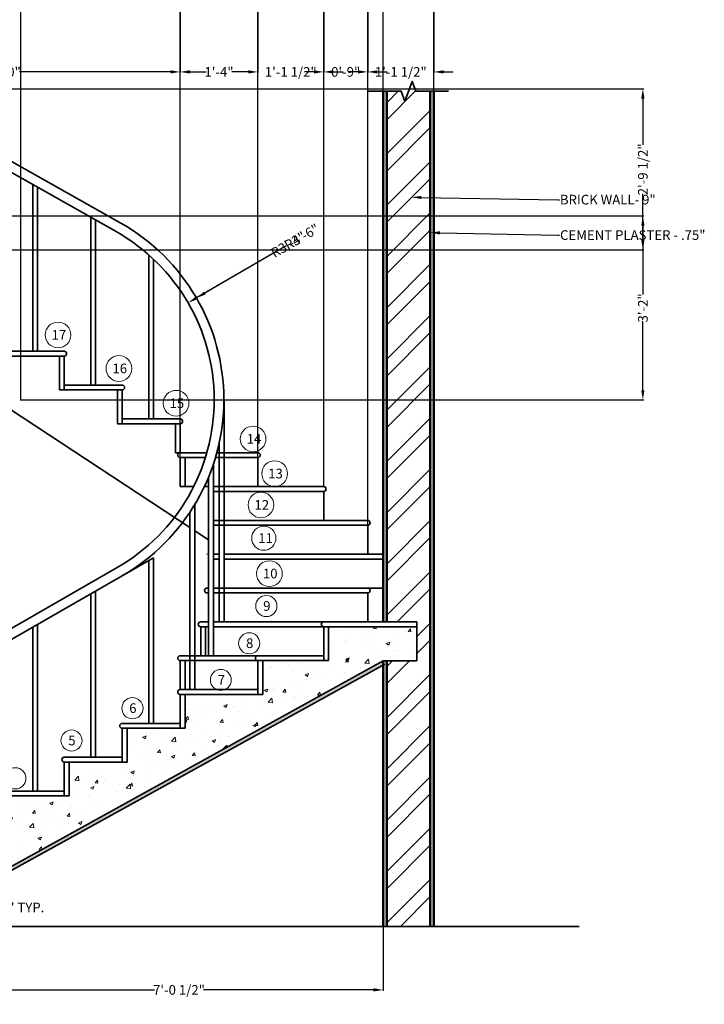
# Model space of a CAD drawing. Units: inches. Extents: x 865 to 1137, y 672 to 989.
# Tile 2 of 3: x 995 to 1137, y 672 to 876. Entities that reach past the tile are written whole.
import ezdxf
from ezdxf import colors
from ezdxf.entities.mleader import LeaderData, LeaderLine
from ezdxf.math import Vec2, Vec3

# ---------------------------------------------------------------- set-up
doc = ezdxf.new("R2010")
doc.units = ezdxf.units.IN
doc.header["$LTSCALE"] = 0.1
doc.header["$MEASUREMENT"] = 0
for name, color, linetype, lineweight in [('A-ANNO-DIMS', 2, 'Continuous', 18), ('A-ANNO-SYMB', 3, 'Continuous', 18), ('A-ANNO-TEXT', 3, 'Continuous', 18), ('A-SECT', 7, 'Continuous', 35), ('A-SECT-PATT', 8, 'Continuous', 13), ('A-WALL', 7, 'Continuous', 50), ('A-WALL-PATT', 8, 'Continuous', 18)]:
    doc.layers.add(name, color=color, linetype=linetype, lineweight=lineweight)
doc.styles.get("Standard").update_dxf_attribs({"font": 'arial.ttf', "height": 2})
doc.dimstyles.get("Standard").update_dxf_attribs({"dimtxt": 2, "dimasz": 2, "dimexe": 0.18, "dimexo": 0.0625, "dimgap": 0.09, "dimtad": 0, "dimdec": 0, "dimzin": 0, "dimdsep": 46, "dimlunit": 3, "dimtxsty": 'Standard', "dimcen": 0.09, "dimadec": 0, "dimazin": 0, "dimtfac": 1, "dimtdec": 0, "dimtofl": 0, "dimtmove": 0, "dimatfit": 3, "dimfxl": 1, "dimtolj": 1, "dimtzin": 0, "dimarcsym": 0})
pattern_1 = [(50, (0, 0), (2.8690407, -0.2510085), [0.3, -3.3]), (355, (0, 0), (-0.5550053, 3.0087685), [0.24, -2.64]), (100.45144, (0.239, -0.021), (2.3140354, 2.75776), [0.254961, -2.8045684]), (46.1842, (0, 0.8), (4.268965, -0.662077), [0.45, -4.95]), (96.63564, (0.3557, 0.745), (3.738648, 3.896474), [0.382441, -4.206855]), (351.18416, (0, 0.8), (3.738648, 3.896474), [0.36, -3.96]), (21, (0.4, 0.6), (2.3876282, -1.6104756), [0.3, -3.3]), (326, (0.4, 0.6), (0.9732613, 2.9006), [0.24, -2.64]), (71.45144, (0.599, 0.4658), (3.3608895, 1.2901246), [0.254961, -2.8045684]), (37.5, (0, 0), (0.0486394, 1.3315754), [0, -2.608, 0, -2.68, 0, -2.65]), (7.5, (0, 0), (1.0522781, 1.5776468), [0, -1.528, 0, -2.548, 0, -1.01]), (327.5, (-0.892, 0), (2.13528974, -0.0902195), [0, -1, 0, -3.12, 0, -4.14]), (317.5, (-1.292, 0), (2.3327447, 0.40042), [0, -1.3, 0, -2.072, 0, -2.94])]

# ---------------------------------------------------------------- blocks, each defined once
blk = doc.blocks.new('STAIR-STEP-SECT')
for p, q in [((13.5, 7), (13.5, 14)), ((0.5, 8), (12.5, 8)), ((0.5, 0), (0.5, 7)), ((0.5, 7), (13.5, 7))]:
    blk.add_line(p, q)
blk.add_arc((0.5, 7.5), 0.5, 90, 270)
blk = doc.blocks.new('*D10')
at = {"layer": 'A-ANNO-DIMS', "color": 0, "lineweight": -2, "transparency": 16777216}
for p, q in [((967.86, 694.49), (967.86, 692.27)), ((981.36, 694.49), (981.36, 692.27)), ((969.86, 692.45), (979.36, 692.45)), ((981.36, 692.45), (983.36, 692.45))]:
    blk.add_line(p, q, dxfattribs=at)
at = {"layer": 'A-ANNO-DIMS', "color": 0, "transparency": 16777216}
for points in [[(969.86, 692.79), (969.86, 692.12), (967.86, 692.45)], [(979.36, 692.79), (979.36, 692.12), (981.36, 692.45)]]:
    blk.add_solid(points, dxfattribs=at)
at = {"layer": 'Defpoints', "color": 0, "transparency": 16777216}
for p in [(967.86, 694.55), (981.36, 694.55), (981.36, 692.45)]:
    blk.add_point(p, dxfattribs=at)
at = {"layer": 'A-ANNO-DIMS', "color": 0, "transparency": 16777216, "insert": (991.78, 692.45), "char_height": 2, "attachment_point": 5}
blk.add_mtext('\\A1;1\'-1 1/2" TYP.', dxfattribs=at)
blk = doc.blocks.new('*D13')
at = {"layer": 'A-ANNO-DIMS', "color": 0, "lineweight": -2, "transparency": 16777216}
for p, q in [((956.36, 891.19), (956.36, 865.17)), ((1028.36, 880.69), (1028.36, 865.17)), ((958.36, 865.35), (989.6, 865.35)), ((1026.36, 865.35), (995.11, 865.35))]:
    blk.add_line(p, q, dxfattribs=at)
at = {"layer": 'A-ANNO-DIMS', "color": 0, "transparency": 16777216}
for points in [[(958.36, 865.69), (958.36, 865.02), (956.36, 865.35)], [(1026.36, 865.69), (1026.36, 865.02), (1028.36, 865.35)]]:
    blk.add_solid(points, dxfattribs=at)
at = {"layer": 'Defpoints', "color": 0, "transparency": 16777216}
for p in [(956.36, 891.25), (1028.36, 880.75), (1028.36, 865.35)]:
    blk.add_point(p, dxfattribs=at)
at = {"layer": 'A-ANNO-DIMS', "color": 0, "transparency": 16777216, "insert": (992.36, 865.35), "char_height": 2, "attachment_point": 5}
blk.add_mtext('\\A1;6\'-0"', dxfattribs=at)
blk = doc.blocks.new('*D14')
at = {"layer": 'A-ANNO-DIMS', "color": 0, "lineweight": -2, "transparency": 16777216}
for p, q in [((1044.43, 894.39), (1044.43, 865.17)), ((1028.36, 880.69), (1028.36, 865.17)), ((1030.36, 865.35), (1033.74, 865.35)), ((1042.43, 865.35), (1039.05, 865.35))]:
    blk.add_line(p, q, dxfattribs=at)
at = {"layer": 'A-ANNO-DIMS', "color": 0, "transparency": 16777216}
for points in [[(1030.36, 865.69), (1030.36, 865.02), (1028.36, 865.35)], [(1042.43, 865.69), (1042.43, 865.02), (1044.43, 865.35)]]:
    blk.add_solid(points, dxfattribs=at)
at = {"layer": 'Defpoints', "color": 0, "transparency": 16777216}
for p in [(1044.43, 894.45), (1028.36, 880.75), (1044.43, 865.35)]:
    blk.add_point(p, dxfattribs=at)
at = {"layer": 'A-ANNO-DIMS', "color": 0, "transparency": 16777216, "insert": (1036.39, 865.35), "char_height": 2, "attachment_point": 5}
blk.add_mtext('\\A1;1\'-4"', dxfattribs=at)
blk = doc.blocks.new('*D15')
at = {"layer": 'A-ANNO-DIMS', "color": 0, "lineweight": -2, "transparency": 16777216}
for p, q in [((1058.06, 903.49), (1058.06, 865.17)), ((1044.43, 894.39), (1044.43, 865.17)), ((1042.43, 865.35), (1040.43, 865.35)), ((1060.06, 865.35), (1062.06, 865.35))]:
    blk.add_line(p, q, dxfattribs=at)
at = {"layer": 'A-ANNO-DIMS', "color": 0, "transparency": 16777216}
for points in [[(1042.43, 865.69), (1042.43, 865.02), (1044.43, 865.35)], [(1060.06, 865.69), (1060.06, 865.02), (1058.06, 865.35)]]:
    blk.add_solid(points, dxfattribs=at)
at = {"layer": 'Defpoints', "color": 0, "transparency": 16777216}
for p in [(1058.06, 903.56), (1044.43, 894.45), (1058.06, 865.35)]:
    blk.add_point(p, dxfattribs=at)
at = {"layer": 'A-ANNO-DIMS', "color": 0, "transparency": 16777216, "insert": (1051.24, 865.35), "char_height": 2, "attachment_point": 5}
blk.add_mtext('\\A1;1\'-1 1/2"', dxfattribs=at)
blk = doc.blocks.new('*D16')
at = {"layer": 'A-ANNO-DIMS', "color": 0, "lineweight": -2, "transparency": 16777216}
for p, q in [((1067.16, 917.12), (1067.16, 865.17)), ((1058.06, 903.49), (1058.06, 865.17)), ((1056.06, 865.35), (1054.06, 865.35)), ((1069.16, 865.35), (1071.16, 865.35))]:
    blk.add_line(p, q, dxfattribs=at)
at = {"layer": 'A-ANNO-DIMS', "color": 0, "transparency": 16777216}
for points in [[(1056.06, 865.69), (1056.06, 865.02), (1058.06, 865.35)], [(1069.16, 865.69), (1069.16, 865.02), (1067.16, 865.35)]]:
    blk.add_solid(points, dxfattribs=at)
at = {"layer": 'Defpoints', "color": 0, "transparency": 16777216}
for p in [(1067.16, 917.18), (1058.06, 903.56), (1067.16, 865.35)]:
    blk.add_point(p, dxfattribs=at)
at = {"layer": 'A-ANNO-DIMS', "color": 0, "transparency": 16777216, "insert": (1062.61, 865.35), "char_height": 2, "attachment_point": 5}
blk.add_mtext('\\A1;0\'-9"', dxfattribs=at)
blk = doc.blocks.new('*D17')
at = {"layer": 'A-ANNO-DIMS', "color": 0, "lineweight": -2, "transparency": 16777216}
for p, q in [((1080.86, 933.19), (1080.86, 865.17)), ((1067.16, 917.12), (1067.16, 865.17)), ((1065.16, 865.35), (1063.16, 865.35)), ((1082.86, 865.35), (1084.86, 865.35))]:
    blk.add_line(p, q, dxfattribs=at)
at = {"layer": 'A-ANNO-DIMS', "color": 0, "transparency": 16777216}
for points in [[(1065.16, 865.69), (1065.16, 865.02), (1067.16, 865.35)], [(1082.86, 865.69), (1082.86, 865.02), (1080.86, 865.35)]]:
    blk.add_solid(points, dxfattribs=at)
at = {"layer": 'Defpoints', "color": 0, "transparency": 16777216}
for p in [(1080.86, 933.25), (1067.16, 917.18), (1080.86, 865.35)]:
    blk.add_point(p, dxfattribs=at)
at = {"layer": 'A-ANNO-DIMS', "color": 0, "transparency": 16777216, "insert": (1074.01, 865.35), "char_height": 2, "attachment_point": 5}
blk.add_mtext('\\A1;1\'-1 1/2"', dxfattribs=at)
blk = doc.blocks.new('*D21')
at = {"layer": 'A-ANNO-DIMS', "color": 0, "lineweight": -2, "transparency": 16777216}
for p, q in [((920.36, 835.61), (920.36, 887.89)), ((922.36, 887.71), (994.85, 887.71)), ((1078.86, 887.71), (1006.37, 887.71)), ((1080.86, 861.4), (1080.86, 887.89))]:
    blk.add_line(p, q, dxfattribs=at)
at = {"layer": 'A-ANNO-DIMS', "color": 0, "transparency": 16777216}
for points in [[(922.36, 888.04), (922.36, 887.37), (920.36, 887.71)], [(1078.86, 888.04), (1078.86, 887.37), (1080.86, 887.71)]]:
    blk.add_solid(points, dxfattribs=at)
at = {"layer": 'Defpoints', "color": 0, "transparency": 16777216}
for p in [(1080.86, 887.71), (1080.86, 861.34), (920.36, 835.55)]:
    blk.add_point(p, dxfattribs=at)
at = {"layer": 'A-ANNO-DIMS', "color": 0, "transparency": 16777216, "insert": (1000.61, 887.71), "char_height": 2, "attachment_point": 5}
blk.add_mtext('\\A1;13\'-4 1/2"', dxfattribs=at)
blk = doc.blocks.new('*D22')
at = {"layer": 'A-ANNO-DIMS', "color": 0, "lineweight": -2, "transparency": 16777216}
for p, q in [((985.86, 709.49), (985.86, 675.22)), ((1070.36, 688.49), (1070.36, 675.22)), ((987.86, 675.4), (1023.04, 675.4)), ((1068.36, 675.4), (1033.18, 675.4))]:
    blk.add_line(p, q, dxfattribs=at)
at = {"layer": 'A-ANNO-DIMS', "color": 0, "transparency": 16777216}
for points in [[(987.86, 675.74), (987.86, 675.07), (985.86, 675.4)], [(1068.36, 675.74), (1068.36, 675.07), (1070.36, 675.4)]]:
    blk.add_solid(points, dxfattribs=at)
at = {"layer": 'Defpoints', "color": 0, "transparency": 16777216}
for p in [(985.86, 709.55), (1070.36, 688.55), (1070.36, 675.4)]:
    blk.add_point(p, dxfattribs=at)
at = {"layer": 'A-ANNO-DIMS', "color": 0, "transparency": 16777216, "insert": (1028.11, 675.4), "char_height": 2, "attachment_point": 5}
blk.add_mtext('\\A1;7\'-0 1/2"', dxfattribs=at)
blk = doc.blocks.new('*D25')
at = {"layer": 'A-ANNO-DIMS', "color": 0, "lineweight": -2, "transparency": 16777216}
for p, q in [((962.92, 861.84), (1124.29, 861.84)), ((1124.11, 859.84), (1124.11, 850.29)), ((1124.11, 830.55), (1124.11, 840.1)), ((962.92, 828.55), (1124.29, 828.55))]:
    blk.add_line(p, q, dxfattribs=at)
at = {"layer": 'A-ANNO-DIMS', "color": 0, "transparency": 16777216}
for points in [[(1123.78, 859.84), (1124.44, 859.84), (1124.11, 861.84)], [(1123.78, 830.55), (1124.44, 830.55), (1124.11, 828.55)]]:
    blk.add_solid(points, dxfattribs=at)
at = {"layer": 'Defpoints', "color": 0, "transparency": 16777216}
for p in [(962.86, 861.84), (1124.11, 861.84), (962.86, 828.55)]:
    blk.add_point(p, dxfattribs=at)
at = {"layer": 'A-ANNO-DIMS', "color": 0, "transparency": 16777216, "insert": (1124.11, 845.19), "char_height": 2, "attachment_point": 5, "rotation": 90}
blk.add_mtext('\\A1;2\'-9 1/2"', dxfattribs=at)
blk = doc.blocks.new('*D30')
at = {"layer": 'A-ANNO-DIMS', "color": 0, "lineweight": -2, "transparency": 16777216}
for p, q in [((995.4, 797.55), (995.4, 887.89)), ((997.4, 887.71), (1030.12, 887.71)), ((1068.36, 887.71), (1035.63, 887.71)), ((1070.36, 861.4), (1070.36, 887.89))]:
    blk.add_line(p, q, dxfattribs=at)
at = {"layer": 'A-ANNO-DIMS', "color": 0, "transparency": 16777216}
for points in [[(997.4, 888.04), (997.4, 887.37), (995.4, 887.71)], [(1068.36, 888.04), (1068.36, 887.37), (1070.36, 887.71)]]:
    blk.add_solid(points, dxfattribs=at)
at = {"layer": 'Defpoints', "color": 0, "transparency": 16777216}
for p in [(1070.36, 887.71), (1070.36, 861.34), (995.4, 797.49)]:
    blk.add_point(p, dxfattribs=at)
at = {"layer": 'A-ANNO-DIMS', "color": 0, "transparency": 16777216, "insert": (1032.88, 887.71), "char_height": 2, "attachment_point": 5}
blk.add_mtext('\\A1;6\'-3"', dxfattribs=at)
blk = doc.blocks.new('*D31')
at = {"layer": 'A-ANNO-DIMS', "color": 0, "lineweight": -2, "transparency": 16777216}
for p, q in [((946.81, 835.55), (1124.29, 835.55)), ((1124.11, 833.55), (1124.11, 819.27)), ((1124.11, 799.49), (1124.11, 813.77)), ((995.46, 797.49), (1124.29, 797.49))]:
    blk.add_line(p, q, dxfattribs=at)
at = {"layer": 'A-ANNO-DIMS', "color": 0, "transparency": 16777216}
for points in [[(1123.78, 833.55), (1124.44, 833.55), (1124.11, 835.55)], [(1123.78, 799.49), (1124.44, 799.49), (1124.11, 797.49)]]:
    blk.add_solid(points, dxfattribs=at)
at = {"layer": 'Defpoints', "color": 0, "transparency": 16777216}
for p in [(946.74, 835.55), (1124.11, 835.55), (995.4, 797.49)]:
    blk.add_point(p, dxfattribs=at)
at = {"layer": 'A-ANNO-DIMS', "color": 0, "transparency": 16777216, "insert": (1124.11, 816.52), "char_height": 2, "attachment_point": 5, "rotation": 90}
blk.add_mtext('\\A1;3\'-2"', dxfattribs=at)
blk = doc.blocks.new('*D32')
at = {"layer": 'A-ANNO-DIMS', "color": 0, "lineweight": -2, "transparency": 16777216}
for p, q in [((1028.36, 779.61), (1028.36, 887.89)), ((1030.36, 887.71), (1033.74, 887.71)), ((1042.43, 887.71), (1039.05, 887.71)), ((1044.43, 779.61), (1044.43, 887.89))]:
    blk.add_line(p, q, dxfattribs=at)
at = {"layer": 'A-ANNO-DIMS', "color": 0, "transparency": 16777216}
for points in [[(1030.36, 888.04), (1030.36, 887.37), (1028.36, 887.71)], [(1042.43, 888.04), (1042.43, 887.37), (1044.43, 887.71)]]:
    blk.add_solid(points, dxfattribs=at)
at = {"layer": 'Defpoints', "color": 0, "transparency": 16777216}
for p in [(1044.43, 887.71), (1028.36, 779.55), (1044.43, 779.55)]:
    blk.add_point(p, dxfattribs=at)
at = {"layer": 'A-ANNO-DIMS', "color": 0, "transparency": 16777216, "insert": (1036.39, 887.71), "char_height": 2, "attachment_point": 5}
blk.add_mtext('\\A1;1\'-4"', dxfattribs=at)
blk = doc.blocks.new('*D33')
at = {"layer": 'A-ANNO-DIMS', "color": 0, "lineweight": -2, "transparency": 16777216}
for p, q in [((1042.43, 887.71), (1040.43, 887.71)), ((1044.43, 785.61), (1044.43, 887.89)), ((1058.06, 779.61), (1058.06, 887.89)), ((1060.06, 887.71), (1062.06, 887.71))]:
    blk.add_line(p, q, dxfattribs=at)
at = {"layer": 'A-ANNO-DIMS', "color": 0, "transparency": 16777216}
for points in [[(1042.43, 888.04), (1042.43, 887.37), (1044.43, 887.71)], [(1060.06, 888.04), (1060.06, 887.37), (1058.06, 887.71)]]:
    blk.add_solid(points, dxfattribs=at)
at = {"layer": 'Defpoints', "color": 0, "transparency": 16777216}
for p in [(1058.06, 887.71), (1044.43, 785.55), (1058.06, 779.55)]:
    blk.add_point(p, dxfattribs=at)
at = {"layer": 'A-ANNO-DIMS', "color": 0, "transparency": 16777216, "insert": (1051.24, 887.71), "char_height": 2, "attachment_point": 5}
blk.add_mtext('\\A1;1\'-1 1/2"', dxfattribs=at)
blk = doc.blocks.new('*D34')
at = {"layer": 'A-ANNO-DIMS', "color": 0, "lineweight": -2, "transparency": 16777216}
for p, q in [((1056.06, 887.71), (1054.06, 887.71)), ((1058.06, 779.61), (1058.06, 887.89)), ((1067.16, 771.61), (1067.16, 887.89)), ((1069.16, 887.71), (1071.16, 887.71))]:
    blk.add_line(p, q, dxfattribs=at)
at = {"layer": 'A-ANNO-DIMS', "color": 0, "transparency": 16777216}
for points in [[(1056.06, 888.04), (1056.06, 887.37), (1058.06, 887.71)], [(1069.16, 888.04), (1069.16, 887.37), (1067.16, 887.71)]]:
    blk.add_solid(points, dxfattribs=at)
at = {"layer": 'Defpoints', "color": 0, "transparency": 16777216}
for p in [(1067.16, 887.71), (1058.06, 779.55), (1067.16, 771.55)]:
    blk.add_point(p, dxfattribs=at)
at = {"layer": 'A-ANNO-DIMS', "color": 0, "transparency": 16777216, "insert": (1062.61, 887.71), "char_height": 2, "attachment_point": 5}
blk.add_mtext('\\A1;0\'-9"', dxfattribs=at)
blk = doc.blocks.new('*D35')
at = {"layer": 'A-ANNO-DIMS', "color": 0, "lineweight": -2, "transparency": 16777216}
for p, q in [((1065.16, 887.71), (1063.16, 887.71)), ((1067.16, 771.61), (1067.16, 887.89)), ((1070.36, 765.61), (1070.36, 887.89)), ((1072.36, 887.71), (1074.36, 887.71))]:
    blk.add_line(p, q, dxfattribs=at)
at = {"layer": 'A-ANNO-DIMS', "color": 0, "transparency": 16777216}
for points in [[(1065.16, 888.04), (1065.16, 887.37), (1067.16, 887.71)], [(1072.36, 888.04), (1072.36, 887.37), (1070.36, 887.71)]]:
    blk.add_solid(points, dxfattribs=at)
at = {"layer": 'Defpoints', "color": 0, "transparency": 16777216}
for p in [(1070.36, 887.71), (1067.16, 771.55), (1070.36, 765.55)]:
    blk.add_point(p, dxfattribs=at)
at = {"layer": 'A-ANNO-DIMS', "color": 0, "transparency": 16777216, "insert": (1077.11, 887.71), "char_height": 2, "attachment_point": 5}
blk.add_mtext('\\A1;0\'-3"', dxfattribs=at)
blk = doc.blocks.new('*D42')
at = {"layer": 'A-ANNO-DIMS', "color": 0, "lineweight": -2, "transparency": 16777216}
for p, q in [((1050.31, 829.36), (1033.45, 819.58)), ((995.31, 797.49), (995.49, 797.49)), ((995.4, 797.4), (995.4, 797.58))]:
    blk.add_line(p, q, dxfattribs=at)
at = {"layer": 'A-ANNO-DIMS', "color": 0, "transparency": 16777216}
blk.add_solid([(1033.28, 819.86), (1033.62, 819.29), (1031.72, 818.57)], dxfattribs=at)
at = {"layer": 'Defpoints', "color": 0, "transparency": 16777216}
for p in [(1031.72, 818.57), (995.4, 797.49)]:
    blk.add_point(p, dxfattribs=at)
at = {"layer": 'A-ANNO-DIMS', "color": 0, "transparency": 16777216, "insert": (1053.51, 831.22), "char_height": 2, "attachment_point": 5, "rotation": 30.1349}
blk.add_mtext('\\A1;R3\'-6"', dxfattribs=at)
blk = doc.blocks.new('*D43')
at = {"layer": 'A-ANNO-DIMS', "color": 0, "lineweight": -2, "transparency": 16777216}
for p, q in [((1047.54, 827.76), (1031.72, 818.57)), ((995.31, 797.49), (995.49, 797.49)), ((995.4, 797.4), (995.4, 797.58))]:
    blk.add_line(p, q, dxfattribs=at)
at = {"layer": 'A-ANNO-DIMS', "color": 0, "transparency": 16777216}
blk.add_solid([(1031.55, 818.86), (1031.89, 818.29), (1029.99, 817.57)], dxfattribs=at)
at = {"layer": 'Defpoints', "color": 0, "transparency": 16777216}
for p in [(1029.99, 817.57), (995.4, 797.49)]:
    blk.add_point(p, dxfattribs=at)
at = {"layer": 'A-ANNO-DIMS', "color": 0, "transparency": 16777216, "insert": (1050.74, 829.62), "char_height": 2, "attachment_point": 5, "rotation": 30.1402}
blk.add_mtext('\\A1;R3\'-4"', dxfattribs=at)

msp = doc.modelspace()

# ---------------------------------------------------------------- hatches: boundary and pattern name
at = {"layer": 'A-SECT-PATT'}
h = msp.add_hatch(dxfattribs=at)
h.set_pattern_fill('AR-CONC', color=256)
h.set_pattern_definition([(50, (0, 0), (7.172602, -0.627521), [0.75, -8.25]), (355, (0, 0), (-1.387513, 7.52192), [0.6, -6.6]), (100.45144, (0.598, -0.052), (5.78509, 6.8944), [0.6374, -7.01142]), (46.1842, (0, 2), (10.672413, -1.65519), [1.125, -12.375]), (96.6356, (0.889, 1.862), (9.34662, 9.74119), [0.9561, -10.51714]), (351.1842, (0, 2), (9.34662, 9.74119), [0.9, -9.9]), (21, (1, 1.5), (5.96907, -4.02619), [0.75, -8.25]), (326, (1, 1.5), (2.433153, 7.2515), [0.6, -6.6]), (71.45144, (1.4974, 1.1645), (8.402224, 3.22531), [0.6374, -7.01142]), (37.5, (0, 0), (0.1215986, 3.3289385), [0, -6.52, 0, -6.7, 0, -6.625]), (7.5, (0, 0), (2.630695, 3.944117), [0, -3.82, 0, -6.37, 0, -2.525]), (327.5, (-2.23, 0), (5.3382244, -0.2255487), [0, -2.5, 0, -7.8, 0, -10.35]), (317.5, (-3.23, 0), (5.831862, 1.00105), [0, -3.25, 0, -5.18, 0, -7.35])])
h.paths.add_polyline_path([(1070.36, 743.46), (1077.35, 743.46), (1077.35, 750.55), (1059.06, 750.55), (1059.06, 743.55), (1045.43, 743.55), (1045.43, 736.55), (1029.36, 736.55), (1029.36, 729.55), (1017.36, 729.55), (1017.36, 722.55), (1005.36, 722.55), (1005.36, 715.55), (993.36, 715.55), (993.36, 708.55), (981.36, 708.55), (981.36, 701.55), (969.36, 701.55), (969.36, 694.55), (957.36, 694.55), (957.36, 688.55), (970.9, 688.55)])
h = msp.add_hatch(dxfattribs=at)
h.set_pattern_fill('AR-CONC', color=256, scale=0.4)
h.set_pattern_definition(pattern_1)
h.paths.add_polyline_path([(1070.36, 742.6), (1070.36, 743.46), (970.9, 688.55), (972.46, 688.55)])
at = {"layer": 'A-WALL-PATT'}
h = msp.add_hatch(dxfattribs=at)
h.set_pattern_fill('ANSI32', color=256, scale=20)
h.paths.add_polyline_path([(1080.11, 861.34), (1077.11, 861.34), (1076.36, 863.4), (1074.86, 859.28), (1074.11, 861.34), (1071.11, 861.34), (1071.11, 751.55), (1077.35, 751.55), (1077.35, 743.46), (1071.11, 743.46), (1071.11, 688.55), (1080.11, 688.55)])
h = msp.add_hatch(dxfattribs=at)
h.set_pattern_fill('AR-CONC', color=256, scale=0.4)
h.set_pattern_definition(pattern_1)
h.paths.add_polyline_path([(1071.11, 743.46), (1070.36, 743.46), (1070.36, 688.55), (1071.11, 688.55)])
h.paths.add_polyline_path([(1071.11, 861.34), (1070.36, 861.34), (1070.36, 751.55), (1071.11, 751.55)])
h.paths.add_polyline_path([(1080.86, 861.34), (1080.11, 861.34), (1080.11, 688.55), (1080.86, 688.55)])

# ---------------------------------------------------------------- linework, layer by layer
at = {"layer": 'A-ANNO-SYMB'}
for centre, radius in [((1003.08, 810.92), 2.66), ((1015.68, 803.98), 2.67), ((1027.5, 796.78), 2.67), ((1043.45, 789.41), 2.65), ((1047.91, 782.22), 2.67), ((1045.06, 775.76), 2.65), ((1045.66, 768.87), 2.51), ((1046.82, 761.53), 2.67), ((1046.19, 754.82), 2.19), ((1042.64, 747.12), 2.19), ((1036.77, 739.54), 2.17), ((1018.47, 733.68), 2.19), ((1005.86, 727), 2.19), ((994.23, 719.18), 2.2)]:
    msp.add_circle(centre, radius, dxfattribs=at)
at = {"layer": 'A-SECT'}
for p, q in [((949.74, 871.55), (1016.07, 834.04)), ((948.76, 869.81), (1015.09, 832.3)), ((997.86, 842.05), (997.86, 807.55)), ((998.86, 807.55), (998.86, 841.48)), ((1009.86, 835.26), (1009.86, 800.55)), ((1010.86, 800.55), (1010.86, 834.69)), ((942.92, 828.55), (1030.37, 771.05)), ((1021.86, 827.48), (1021.86, 793.55)), ((1022.86, 793.55), (1022.86, 826.57)), ((1015.36, 792.55), (1015.36, 799.55)), ((1035.39, 797.88), (1035.39, 797.09)), ((1037.45, 751.55), (1037.45, 797.35)), ((1028.36, 792.55), (1015.36, 792.55)), ((1028.36, 793.55), (1016.36, 793.55)), ((1027.36, 786.55), (1027.36, 792.55)), ((1028.36, 786.55), (1028.36, 792.55)), ((1036.45, 788.63), (1036.45, 751.55)), ((1027.36, 786.55), (1033.87, 786.55)), ((1035.95, 786.55), (1040.28, 786.55)), ((1040.28, 786.55), (1044.43, 786.55)), ((1028.36, 779.55), (1028.36, 785.55)), ((1028.36, 785.55), (1033.58, 785.55)), ((1029.36, 779.55), (1029.36, 785.55)), ((1035.67, 785.55), (1040.28, 785.55)), ((1040.28, 785.55), (1044.43, 785.55)), ((1044.43, 785.55), (1044.43, 779.55)), ((1035.22, 757.55), (1035.22, 784.14)), ((1034.22, 781.46), (1034.22, 744.55)), ((1028.36, 779.55), (1031.15, 779.55)), ((1033.38, 779.55), (1034.22, 779.55)), ((1035.22, 779.55), (1058.06, 779.55)), ((1035.22, 779.55), (1038.29, 779.55)), ((1035.22, 778.55), (1058.06, 778.55)), ((1035.22, 778.55), (1037.29, 778.55)), ((1036.89, 778.55), (1037.55, 778.55)), ((1038.55, 779.55), (1039.28, 779.55)), ((1038.55, 778.55), (1039.28, 778.55)), ((1058.06, 772.55), (1058.06, 778.55)), ((1030.37, 774.23), (1030.37, 737.55)), ((1031.37, 737.55), (1031.37, 775.81)), ((1035.22, 772.55), (1058.06, 772.55)), ((1036.89, 772.55), (1037.55, 772.55)), ((1038.55, 772.55), (1039.28, 772.55)), ((1040.28, 772.55), (1067.16, 772.55)), ((1031.37, 770.39), (1034.22, 768.52)), ((1035.22, 771.55), (1035.89, 771.55)), ((1035.22, 771.55), (1067.16, 771.55)), ((1036.89, 771.55), (1037.55, 771.55)), ((1038.55, 771.55), (1039.28, 771.55)), ((1067.16, 765.55), (1067.16, 771.55)), ((963.86, 730.97), (1022.85, 764.82)), ((1021.86, 764.25), (1021.86, 730.55)), ((1022.86, 730.55), (1022.86, 764.82)), ((1033.9, 765.55), (1033.95, 765.55)), ((1035.22, 765.55), (1035.89, 765.55)), ((1035.22, 765.55), (1036.45, 765.55)), ((1035.22, 764.55), (1035.89, 764.55)), ((1035.22, 764.55), (1036.45, 764.55)), ((1037.45, 765.55), (1037.55, 765.55)), ((1037.45, 765.55), (1070.36, 765.55)), ((1037.45, 764.55), (1037.55, 764.55)), ((1037.45, 764.55), (1070.36, 764.55)), ((1038.55, 765.55), (1039.28, 765.55)), ((1038.55, 764.55), (1039.28, 764.55)), ((963.85, 733.27), (1015.3, 762.79)), ((1010.86, 723.55), (1010.86, 757.93)), ((1033.9, 758.55), (1033.95, 758.55)), ((1033.9, 758.55), (1034.22, 758.55)), ((1035.22, 758.55), (1037.29, 758.55)), ((1036.89, 758.55), (1070.36, 758.55)), ((1009.86, 757.36), (1009.86, 723.55)), ((1033.9, 757.55), (1033.95, 757.55)), ((1033.9, 757.55), (1034.22, 757.55)), ((1035.22, 744.55), (1035.22, 757.55)), ((1035.22, 757.55), (1037.29, 757.55)), ((1036.89, 757.55), (1067.16, 757.55)), ((1067.16, 757.55), (1067.16, 751.55)), ((997.86, 750.48), (997.86, 716.55)), ((998.86, 716.55), (998.86, 751.05)), ((1032.6, 751.55), (1034.22, 751.55)), ((1032.6, 744.55), (1032.6, 750.55)), ((1032.6, 750.55), (1034.22, 750.55)), ((1033.6, 744.55), (1033.6, 750.55)), ((1035.22, 751.55), (1037.29, 751.55)), ((1035.22, 750.55), (1058.06, 750.55)), ((1036.89, 751.55), (1058.06, 751.55)), ((1036.89, 750.55), (1058.06, 750.55)), ((1058.06, 751.55), (1070.36, 751.55)), ((1058.06, 743.55), (1058.06, 750.55)), ((1058.06, 750.55), (1077.35, 750.55)), ((1059.06, 743.55), (1059.06, 750.55)), ((1070.36, 751.55), (1077.35, 751.55)), ((1077.35, 751.55), (1077.35, 743.46)), ((1028.36, 744.55), (1044.43, 744.55)), ((1044.43, 744.55), (1058.06, 744.55)), ((970.9, 688.55), (1070.36, 743.46)), ((972.46, 688.55), (1070.72, 742.8)), ((1028.36, 737.55), (1028.36, 743.55)), ((1028.36, 743.55), (1044.43, 743.55)), ((1029.36, 737.55), (1029.36, 743.55)), ((1044.43, 736.55), (1044.43, 743.55)), ((1044.43, 743.55), (1059.06, 743.55)), ((1045.43, 736.55), (1045.43, 743.55)), ((1070.36, 743.46), (1077.35, 743.46)), ((1028.36, 737.55), (1044.43, 737.55)), ((1028.36, 729.55), (1028.36, 736.55)), ((1028.36, 736.55), (1045.43, 736.55)), ((1110.96, 688.55), (879.61, 688.55))]:
    msp.add_line(p, q, dxfattribs=at)
msp.add_lwpolyline([(1067.36, 861.34), (1074.11, 861.34), (1074.86, 859.28), (1076.36, 863.4), (1077.11, 861.34), (1083.86, 861.34)], dxfattribs=at)
for centre, radius, start, end in [((995.4, 797.49), 42, 299.8461, 60.5124), ((995.4, 797.49), 40, 299.8461, 60.5124), ((1028.36, 793.05), 0.5, 270, 90), ((1028.36, 786.05), 0.5, 90, 270), ((1044.43, 786.05), 0.5, 270, 90), ((1058.06, 779.05), 0.5, 270, 450), ((1067.16, 772.05), 0.5, 270, 450), ((1033.9, 758.05), 0.5, 90, 270), ((1067.16, 758.05), 0.5, 270, 90), ((1032.6, 751.05), 0.5, 90, 270), ((1058.06, 751.05), 0.5, 90, 270), ((1028.36, 744.05), 0.5, 90, 270), ((1044.43, 744.05), 0.5, 90, 270), ((1028.36, 737.05), 0.5, 90, 270)]:
    msp.add_arc(centre, radius, start, end, dxfattribs=at)
at = {"layer": 'A-WALL'}
for p, q in [((1070.36, 861.34), (1070.36, 751.55)), ((1071.11, 861.34), (1071.11, 751.55)), ((1080.11, 861.34), (1080.11, 688.55)), ((1080.86, 861.34), (1080.86, 688.55)), ((1070.36, 743.46), (1070.36, 688.55)), ((1071.11, 743.46), (1071.11, 688.55))]:
    msp.add_line(p, q, dxfattribs=at)

# ---------------------------------------------------------------- block references
at = {"layer": 'A-SECT', "extrusion": (0, 0, -1), "zscale": -1}
for p in [(-1004.86, 799.55), (-1016.86, 792.55)]:
    msp.add_blockref('STAIR-STEP-SECT', p, dxfattribs=at)
at = {"layer": 'A-SECT'}
for p in [(1015.86, 722.55), (1003.86, 715.55), (991.86, 708.55)]:
    msp.add_blockref('STAIR-STEP-SECT', p, dxfattribs=at)

# ---------------------------------------------------------------- texts
at = {"layer": 'A-ANNO-TEXT', "char_height": 2, "attachment_point": 1}
for s, insert in [('17', (1001.74, 811.93)), ('16', (1014.34, 805)), ('15', (1026.15, 797.8)), ('14', (1042.11, 790.42)), ('13', (1046.57, 783.24)), ('12', (1043.73, 776.76)), ('11', (1044.52, 769.88)), ('10', (1045.48, 762.55)), ('9', (1045.53, 755.84)), ('8', (1041.98, 748.14)), ('7', (1036.12, 740.54)), ('6', (1017.81, 734.7)), ('5', (1005.19, 728.01))]:
    msp.add_mtext_dynamic_manual_height_columns(s, width=1.0762, gutter_width=10, heights=[0], dxfattribs=dict(at, insert=insert))

# ---------------------------------------------------------------- dimensions: what is measured, and where the dimension line sits
at = {"layer": 'A-ANNO-DIMS'}
for base, p1, p2, picture, middle in [((1080.86, 865.35), (1067.16, 917.18), (1080.86, 933.25), '*D17', (1074.01, 865.35)), ((1067.16, 865.35), (1058.06, 903.56), (1067.16, 917.18), '*D16', (1062.61, 865.35)), ((1058.06, 865.35), (1044.43, 894.45), (1058.06, 903.56), '*D15', (1051.24, 865.35)), ((1044.43, 865.35), (1028.36, 880.75), (1044.43, 894.45), '*D14', (1036.39, 865.35)), ((1080.86, 887.71), (920.36, 835.55), (1080.86, 861.34), '*D21', (1000.61, 887.71)), ((1028.36, 865.35), (956.36, 891.25), (1028.36, 880.75), '*D13', (992.36, 865.35)), ((1058.06, 887.71), (1044.43, 785.55), (1058.06, 779.55), '*D33', (1051.24, 887.71)), ((1070.36, 887.71), (995.4, 797.49), (1070.36, 861.34), '*D30', (1032.88, 887.71)), ((1044.43, 887.71), (1028.36, 779.55), (1044.43, 779.55), '*D32', (1036.39, 887.71)), ((1067.16, 887.71), (1058.06, 779.55), (1067.16, 771.55), '*D34', (1062.61, 887.71)), ((1070.36, 887.71), (1067.16, 771.55), (1070.36, 765.55), '*D35', (1077.11, 887.71)), ((1070.36, 675.4), (985.86, 709.55), (1070.36, 688.55), '*D22', (1028.11, 675.4))]:
    dim = msp.add_linear_dim(base=base, p1=p1, p2=p2, dimstyle='Standard', override={"dimdec": 1, "dimlfac": 1, "dimrnd": 0, "dimzin": 1, "dimdsep": 46, "dimlunit": 4, "dimfrac": 2}, dxfattribs=at)
    dim.commit()
    dim.dimension.update_dxf_attribs({"geometry": picture, "text_midpoint": middle})
for base, p1, p2, picture, middle in [((1124.11, 861.84), (962.86, 828.55), (962.86, 861.84), '*D25', (1124.11, 845.19)), ((1124.11, 835.55), (995.4, 797.49), (946.74, 835.55), '*D31', (1124.11, 816.52))]:
    dim = msp.add_linear_dim(base=base, p1=p1, p2=p2, angle=90, dimstyle='Standard', override={"dimdec": 1, "dimlfac": 1, "dimrnd": 0, "dimzin": 1, "dimdsep": 46, "dimlunit": 4, "dimfrac": 2}, dxfattribs=at)
    dim.commit()
    dim.dimension.update_dxf_attribs({"geometry": picture, "text_midpoint": middle})
for mpoint, picture, middle in [((1031.72, 818.57), '*D42', (1053.51, 831.22)), ((1029.99, 817.57), '*D43', (1050.74, 829.62))]:
    dim = msp.add_radius_dim(center=(995.4, 797.49), mpoint=mpoint, dimstyle='Standard', override={"dimdec": 1, "dimlfac": 1, "dimrnd": 0, "dimzin": 1, "dimdsep": 46, "dimlunit": 4, "dimfrac": 2}, dxfattribs=at)
    dim.commit()
    dim.dimension.update_dxf_attribs({"geometry": picture, "text_midpoint": middle, "dimtype": 164})
dim = msp.add_linear_dim(base=(981.36, 692.45), p1=(967.86, 694.55), p2=(981.36, 694.55), text='<> TYP.', dimstyle='Standard', override={"dimdec": 1, "dimrnd": 0, "dimzin": 1, "dimlunit": 4, "dimfrac": 2}, dxfattribs=at)
dim.commit()
dim.dimension.update_dxf_attribs({"geometry": '*D10', "text_midpoint": (991.78, 692.45)})

# ---------------------------------------------------------------- leaders
at = {"layer": 'A-ANNO-TEXT'}
ml = msp.add_multileader_mtext('Standard', dxfattribs=at)
ml.set_content('BRICK WALL- 9"', color=256)
ml.set_leader_properties()
ml.build(insert=Vec2(0, 0))
ml.multileader.update_dxf_attribs({"dogleg_length": 0.36, "arrow_head_size": 2})
ctx = ml.context
ctx.base_point, ctx.char_height, ctx.arrow_head_size, ctx.landing_gap_size, ctx.plane_origin = Vec3(1106.85, 838.9), 2, 2, 0.09, Vec3(1076.27, 839.41)
notes = []
notes.append((ctx, [(0, (1, 1, 0), (1106.49, 838.9), (1, 0), 0.36, [(0, [(1076.27, 839.41)], 0, [])])]))
ctx.mtext.insert, ctx.mtext.flow_direction = Vec3(1106.94, 839.92), 5
ml = msp.add_multileader_mtext('Standard', dxfattribs=at)
ml.set_content('CEMENT PLASTER - .75"', color=256)
ml.set_leader_properties()
ml.build(insert=Vec2(0, 0))
ml.multileader.update_dxf_attribs({"dogleg_length": 0.36, "arrow_head_size": 2})
ctx = ml.context
ctx.base_point, ctx.char_height, ctx.arrow_head_size, ctx.landing_gap_size, ctx.plane_origin = Vec3(1106.88, 831.57), 2, 2, 0.09, Vec3(1080.11, 832.09)
notes.append((ctx, [(0, (1, 1, 0), (1106.52, 831.57), (1, 0), 0.36, [(0, [(1080.11, 832.09)], 0, [])])]))
ctx.mtext.insert, ctx.mtext.flow_direction = Vec3(1106.97, 832.59), 5
for ctx, leaders in notes:
    for number, flags, end, landing, length, lines in leaders:
        leader = LeaderData()
        leader.index, (leader.has_last_leader_line, leader.has_dogleg_vector, leader.attachment_direction) = number, flags
        leader.last_leader_point, leader.dogleg_vector, leader.dogleg_length = Vec3(end), Vec3(landing), length
        for number, points, colour, breaks in lines:
            line = LeaderLine()
            line.index, line.vertices, line.color, line.breaks = number, Vec3.list(points), colors.encode_raw_color(colour), breaks
            leader.lines.append(line)
        ctx.leaders.append(leader)

doc.saveas('drawing.dxf')
